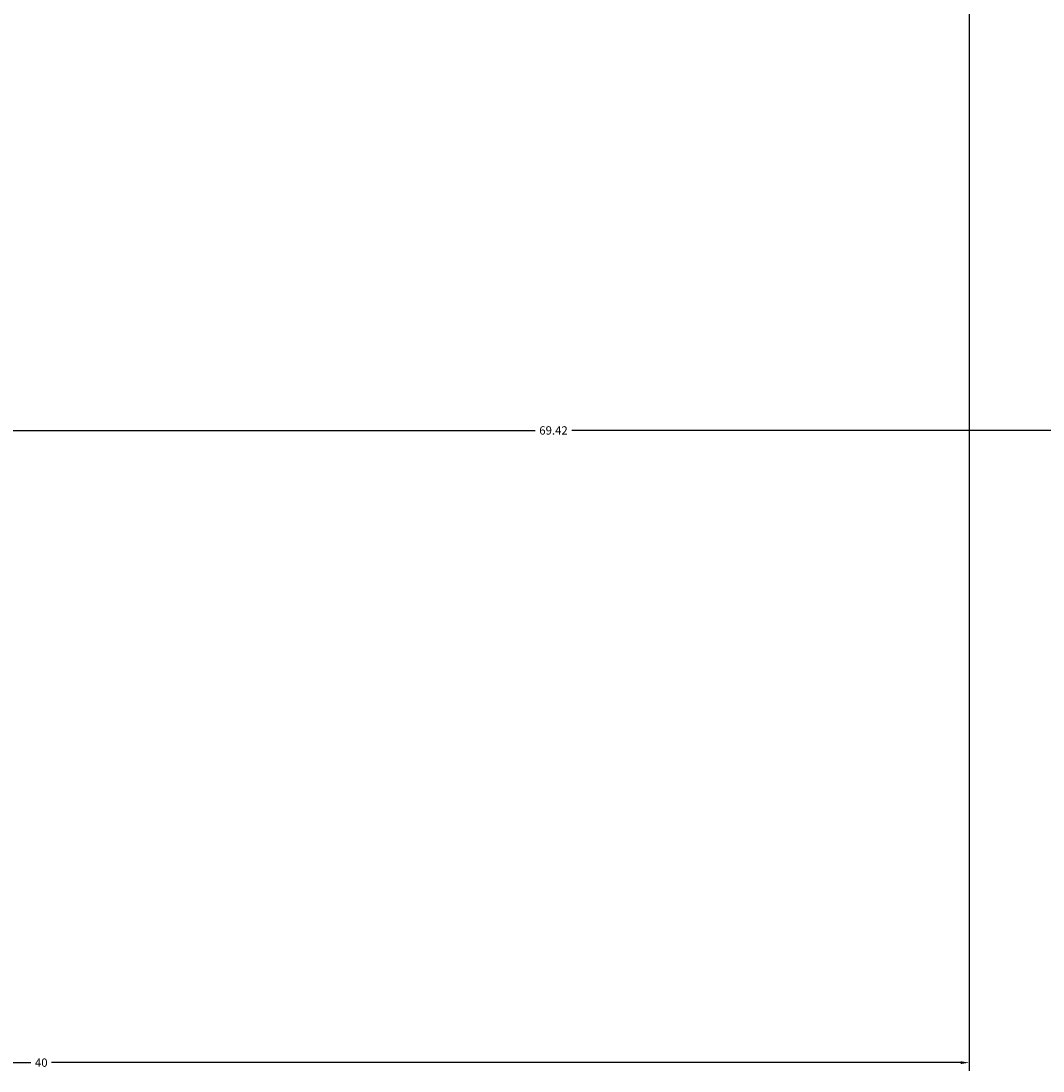
# Model space of a CAD drawing. Units: inches. Extents: x -1 to 292, y -3 to 199.
# Tile 15 of 52: x 102 to 124, y -3 to 20. Entities that reach past the tile are written whole.
import ezdxf

# ---------------------------------------------------------------- set-up
doc = ezdxf.new("R2010")
doc.units = ezdxf.units.IN
doc.header["$MEASUREMENT"] = 0
doc.layers.add('M-DIMS', color=2, linetype='Continuous', lineweight=18)
doc.styles.get("Standard").update_dxf_attribs({"font": 'arial.ttf'})
doc.dimstyles.get("Standard").update_dxf_attribs({"dimtxt": 0.18, "dimasz": 0.18, "dimexe": 0.18, "dimexo": 0.0625, "dimgap": 0.09, "dimtad": 0, "dimtih": 1, "dimtoh": 1, "dimdec": 4, "dimzin": 0, "dimdsep": 46, "dimtxsty": 'Standard', "dimcen": 0.09, "dimadec": 0, "dimazin": 0, "dimtfac": 1, "dimtdec": 4, "dimtofl": 0, "dimtmove": 0, "dimatfit": 3, "dimfxl": 1, "dimtolj": 1, "dimtzin": 0, "dimarcsym": 0})

# ---------------------------------------------------------------- blocks, each defined once
blk = doc.blocks.new('*D13')
at = {"layer": 'Defpoints', "color": 0, "transparency": 16777216}
for p in [(79.013, 25.514), (148.429, 25.514), (79.013, 10.914)]:
    blk.add_point(p, dxfattribs=at)
at = {"layer": 'M-DIMS', "color": 0, "lineweight": -2, "transparency": 16777216}
for p, q in [((79.013, 25.452), (79.013, 10.734)), ((148.429, 25.452), (148.429, 10.734)), ((79.193, 10.914), (113.328, 10.914)), ((148.249, 10.914), (114.115, 10.914))]:
    blk.add_line(p, q, dxfattribs=at)
at = {"layer": 'M-DIMS', "color": 0, "transparency": 16777216}
for points in [[(79.193, 10.944), (79.193, 10.884), (79.013, 10.914)], [(148.249, 10.944), (148.249, 10.884), (148.429, 10.914)]]:
    blk.add_solid(points, dxfattribs=at)
at = {"layer": 'M-DIMS', "color": 0, "transparency": 16777216, "insert": (113.721, 10.914), "char_height": 0.18, "attachment_point": 5}
blk.add_mtext('\\A1;69.42', dxfattribs=at)
blk = doc.blocks.new('*D22')
at = {"layer": 'Defpoints', "color": 0, "transparency": 16777216}
for p in [(82.679, 51.267), (122.679, 51.267), (122.679, -2.71)]:
    blk.add_point(p, dxfattribs=at)
at = {"layer": 'M-DIMS', "color": 0, "lineweight": -2, "transparency": 16777216}
for p, q in [((82.679, 51.205), (82.679, -2.89)), ((122.679, 51.205), (122.679, -2.89)), ((82.859, -2.71), (102.457, -2.71)), ((122.499, -2.71), (102.901, -2.71))]:
    blk.add_line(p, q, dxfattribs=at)
at = {"layer": 'M-DIMS', "color": 0, "transparency": 16777216}
for points in [[(82.859, -2.68), (82.859, -2.74), (82.679, -2.71)], [(122.499, -2.68), (122.499, -2.74), (122.679, -2.71)]]:
    blk.add_solid(points, dxfattribs=at)
at = {"layer": 'M-DIMS', "color": 0, "transparency": 16777216, "insert": (102.679, -2.71), "char_height": 0.18, "attachment_point": 5}
blk.add_mtext('\\A1;40', dxfattribs=at)

msp = doc.modelspace()

# ---------------------------------------------------------------- dimensions: what is measured, and where the dimension line sits
at = {"layer": 'M-DIMS'}
dim = msp.add_linear_dim(base=(122.6788, -2.7104), p1=(82.6788, 51.2672), p2=(122.6788, 51.2672), dimstyle='Standard', override={"dimdec": 0, "dimlfac": 1, "dimrnd": 0, "dimzin": 0, "dimdsep": 46, "dimlunit": 2}, dxfattribs=at)
dim.commit()
dim.dimension.update_dxf_attribs({"geometry": '*D22', "text_midpoint": (102.6788, -2.7104)})
dim = msp.add_linear_dim(base=(79.013, 10.9141), p1=(148.4295, 25.5141), p2=(79.013, 25.5141), angle=180, dimstyle='Standard', override={"dimdec": 2, "dimlfac": 1, "dimrnd": 0, "dimzin": 0, "dimdsep": 46, "dimlunit": 2}, dxfattribs=at)
dim.commit()
dim.dimension.update_dxf_attribs({"geometry": '*D13', "text_midpoint": (113.7212, 10.9141)})

doc.saveas('drawing.dxf')
